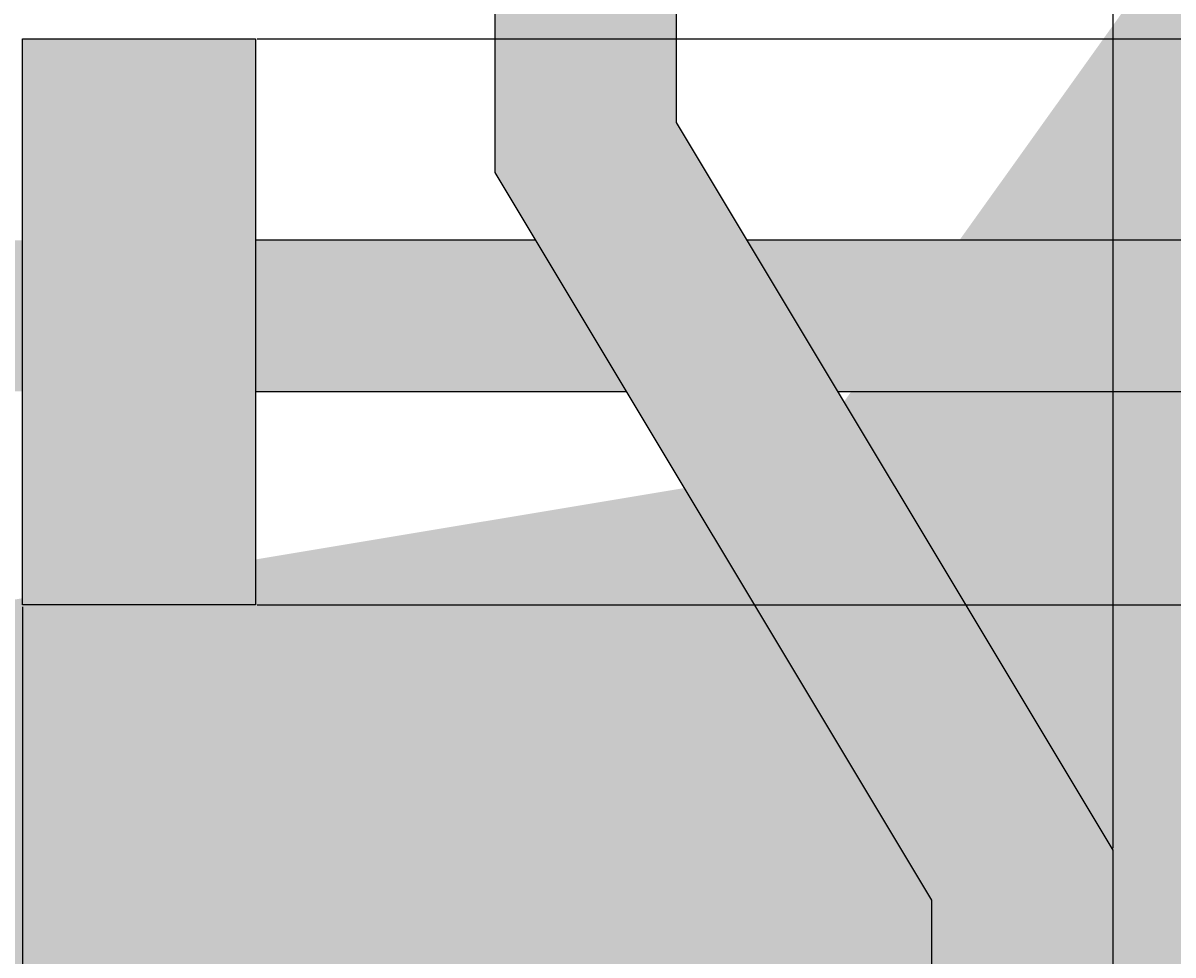
# Model space of a CAD drawing. Units: millimetres. Extents: x -22994 to 29398, y -19990 to 20176.
# Tile 111 of 135: x 166 to 204, y 124 to 155. Entities that reach past the tile are written whole.
import ezdxf

# ---------------------------------------------------------------- set-up
doc = ezdxf.new("R2010")
doc.units = ezdxf.units.MM
doc.header["$MEASUREMENT"] = 0
for name, color, linetype, lineweight in [('M-DIMS', 2, 'Continuous', 18), ('M-EQPM', 7, 'Continuous', 25), ('M-EQPM-PATT', 7, 'Continuous', 18)]:
    doc.layers.add(name, color=color, linetype=linetype, lineweight=lineweight)
doc.styles.get("Standard").update_dxf_attribs({"font": 'arial.ttf'})
doc.dimstyles.get("Standard").update_dxf_attribs({"dimtxt": 0.18, "dimasz": 10000, "dimexe": 0.18, "dimexo": 0.0625, "dimgap": 0.09, "dimtad": 0, "dimtih": 1, "dimtoh": 1, "dimdec": 0, "dimzin": 0, "dimdsep": 46, "dimtxsty": 'Standard', "dimcen": 0.09, "dimadec": 0, "dimazin": 0, "dimtfac": 1, "dimtdec": 0, "dimtofl": 0, "dimtmove": 0, "dimatfit": 3, "dimfxl": 1, "dimtolj": 1, "dimtzin": 0, "dimlwd": 30, "dimarcsym": 0})

# ---------------------------------------------------------------- blocks, each defined once
blk = doc.blocks.new('*D2')
at = {"layer": 'Defpoints', "color": 0, "transparency": 16777216}
for p in [(6.677, 10.271), (290.852, 10.271), (290.852, -5.079)]:
    blk.add_point(p, dxfattribs=at)
at = {"layer": 'M-DIMS', "color": 0, "lineweight": -2, "transparency": 16777216}
for p, q in [((6.677, 10.209), (6.677, -5.259)), ((290.852, 10.209), (290.852, -5.259))]:
    blk.add_line(p, q, dxfattribs=at)
at = {"layer": 'M-DIMS', "color": 0, "lineweight": 30, "transparency": 16777216}
for p, q in [((-9993.323, -5.079), (-19993.323, -5.079)), ((10290.852, -5.079), (20290.852, -5.079))]:
    blk.add_line(p, q, dxfattribs=at)
at = {"layer": 'M-DIMS', "color": 0, "transparency": 16777216}
for points in [[(-9993.323, 1661.588), (-9993.323, -1671.745), (6.677, -5.079)], [(10290.852, 1661.588), (10290.852, -1671.745), (290.852, -5.079)]]:
    blk.add_solid(points, dxfattribs=at)
at = {"layer": 'M-DIMS', "color": 0, "transparency": 16777216, "insert": (148.765, -5.079), "char_height": 0.18, "attachment_point": 5}
blk.add_mtext('\\A1;284.2', dxfattribs=at)
blk = doc.blocks.new('*D3')
at = {"layer": 'Defpoints', "color": 0, "transparency": 16777216}
for p in [(110.265, 204.165), (110.265, 176.366), (95.833, 127.967)]:
    blk.add_point(p, dxfattribs=at)
at = {"layer": 'M-DIMS', "color": 0, "lineweight": 30, "transparency": 16777216}
for p, q in [((-9904.167, 204.165), (-19904.167, 204.165)), ((10110.265, 204.165), (20110.265, 204.165))]:
    blk.add_line(p, q, dxfattribs=at)
at = {"layer": 'M-DIMS', "color": 0, "lineweight": -2, "transparency": 16777216}
for p, q in [((95.833, 128.03), (95.833, 204.345)), ((110.265, 176.429), (110.265, 204.345))]:
    blk.add_line(p, q, dxfattribs=at)
at = {"layer": 'M-DIMS', "color": 0, "transparency": 16777216}
for points in [[(-9904.167, 1870.832), (-9904.167, -1462.501), (95.833, 204.165)], [(10110.265, 1870.832), (10110.265, -1462.501), (110.265, 204.165)]]:
    blk.add_solid(points, dxfattribs=at)
at = {"layer": 'M-DIMS', "color": 0, "transparency": 16777216, "insert": (103.049, 204.165), "char_height": 0.18, "attachment_point": 5}
blk.add_mtext('\\A1;14.432', dxfattribs=at)
blk = doc.blocks.new('*D4')
at = {"layer": 'Defpoints', "color": 0, "transparency": 16777216}
for p in [(116.265, 204.165), (110.265, 176.366), (116.265, 176.366)]:
    blk.add_point(p, dxfattribs=at)
at = {"layer": 'M-DIMS', "color": 0, "lineweight": 30, "transparency": 16777216}
for p, q in [((-9889.735, 204.165), (-19889.735, 204.165)), ((10116.265, 204.165), (20116.265, 204.165))]:
    blk.add_line(p, q, dxfattribs=at)
at = {"layer": 'M-DIMS', "color": 0, "lineweight": -2, "transparency": 16777216}
for p, q in [((110.265, 176.429), (110.265, 204.345)), ((116.265, 176.429), (116.265, 204.345))]:
    blk.add_line(p, q, dxfattribs=at)
at = {"layer": 'M-DIMS', "color": 0, "transparency": 16777216}
for points in [[(-9889.735, 1870.832), (-9889.735, -1462.501), (110.265, 204.165)], [(10116.265, 1870.832), (10116.265, -1462.501), (116.265, 204.165)]]:
    blk.add_solid(points, dxfattribs=at)
at = {"layer": 'M-DIMS', "color": 0, "transparency": 16777216, "insert": (113.265, 204.165), "char_height": 0.18, "attachment_point": 5}
blk.add_mtext('\\A1;6', dxfattribs=at)
blk = doc.blocks.new('*D5')
at = {"layer": 'Defpoints', "color": 0, "transparency": 16777216}
for p in [(181.265, 204.165), (116.265, 176.366), (181.265, 176.366)]:
    blk.add_point(p, dxfattribs=at)
at = {"layer": 'M-DIMS', "color": 0, "lineweight": 30, "transparency": 16777216}
for p, q in [((-9883.735, 204.165), (-19883.735, 204.165)), ((10181.265, 204.165), (20181.265, 204.165))]:
    blk.add_line(p, q, dxfattribs=at)
at = {"layer": 'M-DIMS', "color": 0, "lineweight": -2, "transparency": 16777216}
for p, q in [((116.265, 176.429), (116.265, 204.345)), ((181.265, 176.429), (181.265, 204.345))]:
    blk.add_line(p, q, dxfattribs=at)
at = {"layer": 'M-DIMS', "color": 0, "transparency": 16777216}
for points in [[(-9883.735, 1870.832), (-9883.735, -1462.501), (116.265, 204.165)], [(10181.265, 1870.832), (10181.265, -1462.501), (181.265, 204.165)]]:
    blk.add_solid(points, dxfattribs=at)
at = {"layer": 'M-DIMS', "color": 0, "transparency": 16777216, "insert": (148.765, 204.165), "char_height": 0.18, "attachment_point": 5}
blk.add_mtext('\\A1;65', dxfattribs=at)
blk = doc.blocks.new('*D6')
at = {"layer": 'Defpoints', "color": 0, "transparency": 16777216}
for p in [(187.265, 204.165), (181.265, 176.366), (187.265, 176.366)]:
    blk.add_point(p, dxfattribs=at)
at = {"layer": 'M-DIMS', "color": 0, "lineweight": 30, "transparency": 16777216}
for p, q in [((-9818.735, 204.165), (-19818.735, 204.165)), ((10187.265, 204.165), (20187.265, 204.165))]:
    blk.add_line(p, q, dxfattribs=at)
at = {"layer": 'M-DIMS', "color": 0, "lineweight": -2, "transparency": 16777216}
for p, q in [((181.265, 176.429), (181.265, 204.345)), ((187.265, 176.429), (187.265, 204.345))]:
    blk.add_line(p, q, dxfattribs=at)
at = {"layer": 'M-DIMS', "color": 0, "transparency": 16777216}
for points in [[(-9818.735, 1870.832), (-9818.735, -1462.501), (181.265, 204.165)], [(10187.265, 1870.832), (10187.265, -1462.501), (187.265, 204.165)]]:
    blk.add_solid(points, dxfattribs=at)
at = {"layer": 'M-DIMS', "color": 0, "transparency": 16777216, "insert": (184.265, 204.165), "char_height": 0.18, "attachment_point": 5}
blk.add_mtext('\\A1;6', dxfattribs=at)
blk = doc.blocks.new('*D7')
at = {"layer": 'Defpoints', "color": 0, "transparency": 16777216}
for p in [(201.697, 204.165), (187.265, 176.366), (201.697, 127.967)]:
    blk.add_point(p, dxfattribs=at)
at = {"layer": 'M-DIMS', "color": 0, "lineweight": 30, "transparency": 16777216}
for p, q in [((-9812.735, 204.165), (-19812.735, 204.165)), ((10201.697, 204.165), (20201.697, 204.165))]:
    blk.add_line(p, q, dxfattribs=at)
at = {"layer": 'M-DIMS', "color": 0, "lineweight": -2, "transparency": 16777216}
for p, q in [((187.265, 176.429), (187.265, 204.345)), ((201.697, 128.03), (201.697, 204.345))]:
    blk.add_line(p, q, dxfattribs=at)
at = {"layer": 'M-DIMS', "color": 0, "transparency": 16777216}
for points in [[(-9812.735, 1870.832), (-9812.735, -1462.501), (187.265, 204.165)], [(10201.697, 1870.832), (10201.697, -1462.501), (201.697, 204.165)]]:
    blk.add_solid(points, dxfattribs=at)
at = {"layer": 'M-DIMS', "color": 0, "transparency": 16777216, "insert": (194.481, 204.165), "char_height": 0.18, "attachment_point": 5}
blk.add_mtext('\\A1;14.432', dxfattribs=at)
blk = doc.blocks.new('*D8')
at = {"layer": 'Defpoints', "color": 0, "transparency": 16777216}
for p in [(227.648, 204.165), (227.648, 146.73), (201.697, 127.967)]:
    blk.add_point(p, dxfattribs=at)
at = {"layer": 'M-DIMS', "color": 0, "lineweight": 30, "transparency": 16777216}
for p, q in [((-9798.303, 204.165), (-19798.303, 204.165)), ((10227.648, 204.165), (20227.648, 204.165))]:
    blk.add_line(p, q, dxfattribs=at)
at = {"layer": 'M-DIMS', "color": 0, "lineweight": -2, "transparency": 16777216}
for p, q in [((201.697, 128.03), (201.697, 204.345)), ((227.648, 146.792), (227.648, 204.345))]:
    blk.add_line(p, q, dxfattribs=at)
at = {"layer": 'M-DIMS', "color": 0, "transparency": 16777216}
for points in [[(-9798.303, 1870.832), (-9798.303, -1462.501), (201.697, 204.165)], [(10227.648, 1870.832), (10227.648, -1462.501), (227.648, 204.165)]]:
    blk.add_solid(points, dxfattribs=at)
at = {"layer": 'M-DIMS', "color": 0, "transparency": 16777216, "insert": (214.673, 204.165), "char_height": 0.18, "attachment_point": 5}
blk.add_mtext('\\A1;25.95', dxfattribs=at)
blk = doc.blocks.new('*D9')
at = {"layer": 'Defpoints', "color": 0, "transparency": 16777216}
for p in [(187.265, 176.366), (306.202, 176.366), (290.852, 10.271)]:
    blk.add_point(p, dxfattribs=at)
at = {"layer": 'M-DIMS', "color": 0, "lineweight": 30, "transparency": 16777216}
for p, q in [((306.202, 10176.366), (306.202, 20176.366)), ((306.202, -9989.729), (306.202, -19989.729))]:
    blk.add_line(p, q, dxfattribs=at)
at = {"layer": 'M-DIMS', "color": 0, "lineweight": -2, "transparency": 16777216}
for p, q in [((187.327, 176.366), (306.382, 176.366)), ((290.915, 10.271), (306.382, 10.271))]:
    blk.add_line(p, q, dxfattribs=at)
at = {"layer": 'M-DIMS', "color": 0, "transparency": 16777216}
for points in [[(-1360.465, 10176.366), (1972.869, 10176.366), (306.202, 176.366)], [(-1360.465, -9989.729), (1972.869, -9989.729), (306.202, 10.271)]]:
    blk.add_solid(points, dxfattribs=at)
at = {"layer": 'M-DIMS', "color": 0, "transparency": 16777216, "insert": (306.202, 93.319), "char_height": 0.18, "attachment_point": 5}
blk.add_mtext('\\A1;166.1', dxfattribs=at)
blk = doc.blocks.new('*D10')
at = {"layer": 'Defpoints', "color": 0, "transparency": 16777216}
for p in [(125.65, 136.071), (133.346, 136.071), (133.346, -5.079)]:
    blk.add_point(p, dxfattribs=at)
at = {"layer": 'M-DIMS', "color": 0, "lineweight": -2, "transparency": 16777216}
for p, q in [((125.65, 136.009), (125.65, -5.259)), ((133.346, 136.009), (133.346, -5.259))]:
    blk.add_line(p, q, dxfattribs=at)
at = {"layer": 'M-DIMS', "color": 0, "lineweight": 30, "transparency": 16777216}
for p, q in [((-9874.35, -5.079), (-19874.35, -5.079)), ((10133.346, -5.079), (20133.346, -5.079))]:
    blk.add_line(p, q, dxfattribs=at)
at = {"layer": 'M-DIMS', "color": 0, "transparency": 16777216}
for points in [[(-9874.35, 1661.588), (-9874.35, -1671.745), (125.65, -5.079)], [(10133.346, 1661.588), (10133.346, -1671.745), (133.346, -5.079)]]:
    blk.add_solid(points, dxfattribs=at)
at = {"layer": 'M-DIMS', "color": 0, "transparency": 16777216, "insert": (129.498, -5.079), "char_height": 0.18, "attachment_point": 5}
blk.add_mtext('\\A1;7.696', dxfattribs=at)
blk = doc.blocks.new('*D11')
at = {"layer": 'Defpoints', "color": 0, "transparency": 16777216}
for p in [(133.346, 136.071), (135.65, 136.071), (135.65, -5.079)]:
    blk.add_point(p, dxfattribs=at)
at = {"layer": 'M-DIMS', "color": 0, "lineweight": -2, "transparency": 16777216}
for p, q in [((133.346, 136.009), (133.346, -5.259)), ((135.65, 136.009), (135.65, -5.259))]:
    blk.add_line(p, q, dxfattribs=at)
at = {"layer": 'M-DIMS', "color": 0, "lineweight": 30, "transparency": 16777216}
for p, q in [((-9866.654, -5.079), (-19866.654, -5.079)), ((10135.65, -5.079), (20135.65, -5.079))]:
    blk.add_line(p, q, dxfattribs=at)
at = {"layer": 'M-DIMS', "color": 0, "transparency": 16777216}
for points in [[(-9866.654, 1661.588), (-9866.654, -1671.745), (133.346, -5.079)], [(10135.65, 1661.588), (10135.65, -1671.745), (135.65, -5.079)]]:
    blk.add_solid(points, dxfattribs=at)
at = {"layer": 'M-DIMS', "color": 0, "transparency": 16777216, "insert": (134.498, -5.079), "char_height": 0.18, "attachment_point": 5}
blk.add_mtext('\\A1;2.304', dxfattribs=at)
blk = doc.blocks.new('*D12')
at = {"layer": 'Defpoints', "color": 0, "transparency": 16777216}
for p in [(135.65, 136.071), (145.65, 136.071), (145.65, -5.079)]:
    blk.add_point(p, dxfattribs=at)
at = {"layer": 'M-DIMS', "color": 0, "lineweight": -2, "transparency": 16777216}
for p, q in [((135.65, 136.009), (135.65, -5.259)), ((145.65, 136.009), (145.65, -5.259))]:
    blk.add_line(p, q, dxfattribs=at)
at = {"layer": 'M-DIMS', "color": 0, "lineweight": 30, "transparency": 16777216}
for p, q in [((-9864.35, -5.079), (-19864.35, -5.079)), ((10145.65, -5.079), (20145.65, -5.079))]:
    blk.add_line(p, q, dxfattribs=at)
at = {"layer": 'M-DIMS', "color": 0, "transparency": 16777216}
for points in [[(-9864.35, 1661.588), (-9864.35, -1671.745), (135.65, -5.079)], [(10145.65, 1661.588), (10145.65, -1671.745), (145.65, -5.079)]]:
    blk.add_solid(points, dxfattribs=at)
at = {"layer": 'M-DIMS', "color": 0, "transparency": 16777216, "insert": (140.65, -5.079), "char_height": 0.18, "attachment_point": 5}
blk.add_mtext('\\A1;10', dxfattribs=at)
blk = doc.blocks.new('*D13')
at = {"layer": 'Defpoints', "color": 0, "transparency": 16777216}
for p in [(145.65, 136.071), (155.65, 136.071), (155.65, -5.079)]:
    blk.add_point(p, dxfattribs=at)
at = {"layer": 'M-DIMS', "color": 0, "lineweight": -2, "transparency": 16777216}
for p, q in [((145.65, 136.009), (145.65, -5.259)), ((155.65, 136.009), (155.65, -5.259))]:
    blk.add_line(p, q, dxfattribs=at)
at = {"layer": 'M-DIMS', "color": 0, "lineweight": 30, "transparency": 16777216}
for p, q in [((-9854.35, -5.079), (-19854.35, -5.079)), ((10155.65, -5.079), (20155.65, -5.079))]:
    blk.add_line(p, q, dxfattribs=at)
at = {"layer": 'M-DIMS', "color": 0, "transparency": 16777216}
for points in [[(-9854.35, 1661.588), (-9854.35, -1671.745), (145.65, -5.079)], [(10155.65, 1661.588), (10155.65, -1671.745), (155.65, -5.079)]]:
    blk.add_solid(points, dxfattribs=at)
at = {"layer": 'M-DIMS', "color": 0, "transparency": 16777216, "insert": (150.65, -5.079), "char_height": 0.18, "attachment_point": 5}
blk.add_mtext('\\A1;10', dxfattribs=at)
blk = doc.blocks.new('*D14')
at = {"layer": 'Defpoints', "color": 0, "transparency": 16777216}
for p in [(155.65, 136.071), (165.65, 136.071), (165.65, -5.079)]:
    blk.add_point(p, dxfattribs=at)
at = {"layer": 'M-DIMS', "color": 0, "lineweight": -2, "transparency": 16777216}
for p, q in [((155.65, 136.009), (155.65, -5.259)), ((165.65, 136.009), (165.65, -5.259))]:
    blk.add_line(p, q, dxfattribs=at)
at = {"layer": 'M-DIMS', "color": 0, "lineweight": 30, "transparency": 16777216}
for p, q in [((-9844.35, -5.079), (-19844.35, -5.079)), ((10165.65, -5.079), (20165.65, -5.079))]:
    blk.add_line(p, q, dxfattribs=at)
at = {"layer": 'M-DIMS', "color": 0, "transparency": 16777216}
for points in [[(-9844.35, 1661.588), (-9844.35, -1671.745), (155.65, -5.079)], [(10165.65, 1661.588), (10165.65, -1671.745), (165.65, -5.079)]]:
    blk.add_solid(points, dxfattribs=at)
at = {"layer": 'M-DIMS', "color": 0, "transparency": 16777216, "insert": (160.65, -5.079), "char_height": 0.18, "attachment_point": 5}
blk.add_mtext('\\A1;10', dxfattribs=at)
blk = doc.blocks.new('*D15')
at = {"layer": 'Defpoints', "color": 0, "transparency": 16777216}
for p in [(173.346, 154.788), (173.346, 136.071), (306.202, 136.071)]:
    blk.add_point(p, dxfattribs=at)
at = {"layer": 'M-DIMS', "color": 0, "lineweight": 30, "transparency": 16777216}
for p, q in [((306.202, 10154.788), (306.202, 20154.788)), ((306.202, -9863.929), (306.202, -19863.929))]:
    blk.add_line(p, q, dxfattribs=at)
at = {"layer": 'M-DIMS', "color": 0, "lineweight": -2, "transparency": 16777216}
for p, q in [((173.408, 154.788), (306.382, 154.788)), ((173.408, 136.071), (306.382, 136.071))]:
    blk.add_line(p, q, dxfattribs=at)
at = {"layer": 'M-DIMS', "color": 0, "transparency": 16777216}
for points in [[(-1360.465, 10154.788), (1972.869, 10154.788), (306.202, 154.788)], [(-1360.465, -9863.929), (1972.869, -9863.929), (306.202, 136.071)]]:
    blk.add_solid(points, dxfattribs=at)
at = {"layer": 'M-DIMS', "color": 0, "transparency": 16777216, "insert": (306.202, 145.43), "char_height": 0.18, "attachment_point": 5}
blk.add_mtext('\\A1;18.717', dxfattribs=at)
blk = doc.blocks.new('*D16')
at = {"layer": 'Defpoints', "color": 0, "transparency": 16777216}
for p in [(120.17, 204.165), (110.466, 48.035), (120.17, 48.035)]:
    blk.add_point(p, dxfattribs=at)
at = {"layer": 'M-DIMS', "color": 0, "lineweight": 30, "transparency": 16777216}
for p, q in [((-9889.534, 204.165), (-19889.534, 204.165)), ((10120.17, 204.165), (20120.17, 204.165))]:
    blk.add_line(p, q, dxfattribs=at)
at = {"layer": 'M-DIMS', "color": 0, "lineweight": -2, "transparency": 16777216}
for p, q in [((110.466, 48.097), (110.466, 204.345)), ((120.17, 48.097), (120.17, 204.345))]:
    blk.add_line(p, q, dxfattribs=at)
at = {"layer": 'M-DIMS', "color": 0, "transparency": 16777216}
for points in [[(-9889.534, 1870.832), (-9889.534, -1462.501), (110.466, 204.165)], [(10120.17, 1870.832), (10120.17, -1462.501), (120.17, 204.165)]]:
    blk.add_solid(points, dxfattribs=at)
at = {"layer": 'M-DIMS', "color": 0, "transparency": 16777216, "insert": (115.318, 204.165), "char_height": 0.18, "attachment_point": 5}
blk.add_mtext('\\A1;9.704', dxfattribs=at)
blk = doc.blocks.new('*D17')
at = {"layer": 'Defpoints', "color": 0, "transparency": 16777216}
for p in [(126.17, 204.165), (120.17, 48.035), (126.17, 48.035)]:
    blk.add_point(p, dxfattribs=at)
at = {"layer": 'M-DIMS', "color": 0, "lineweight": 30, "transparency": 16777216}
for p, q in [((-9879.83, 204.165), (-19879.83, 204.165)), ((10126.17, 204.165), (20126.17, 204.165))]:
    blk.add_line(p, q, dxfattribs=at)
at = {"layer": 'M-DIMS', "color": 0, "lineweight": -2, "transparency": 16777216}
for p, q in [((120.17, 48.097), (120.17, 204.345)), ((126.17, 48.097), (126.17, 204.345))]:
    blk.add_line(p, q, dxfattribs=at)
at = {"layer": 'M-DIMS', "color": 0, "transparency": 16777216}
for points in [[(-9879.83, 1870.832), (-9879.83, -1462.501), (120.17, 204.165)], [(10126.17, 1870.832), (10126.17, -1462.501), (126.17, 204.165)]]:
    blk.add_solid(points, dxfattribs=at)
at = {"layer": 'M-DIMS', "color": 0, "transparency": 16777216, "insert": (123.17, 204.165), "char_height": 0.18, "attachment_point": 5}
blk.add_mtext('\\A1;6', dxfattribs=at)
blk = doc.blocks.new('*D18')
at = {"layer": 'Defpoints', "color": 0, "transparency": 16777216}
for p in [(132.17, 204.165), (126.17, 48.035), (132.17, 48.035)]:
    blk.add_point(p, dxfattribs=at)
at = {"layer": 'M-DIMS', "color": 0, "lineweight": 30, "transparency": 16777216}
for p, q in [((-9873.83, 204.165), (-19873.83, 204.165)), ((10132.17, 204.165), (20132.17, 204.165))]:
    blk.add_line(p, q, dxfattribs=at)
at = {"layer": 'M-DIMS', "color": 0, "lineweight": -2, "transparency": 16777216}
for p, q in [((126.17, 48.097), (126.17, 204.345)), ((132.17, 48.097), (132.17, 204.345))]:
    blk.add_line(p, q, dxfattribs=at)
at = {"layer": 'M-DIMS', "color": 0, "transparency": 16777216}
for points in [[(-9873.83, 1870.832), (-9873.83, -1462.501), (126.17, 204.165)], [(10132.17, 1870.832), (10132.17, -1462.501), (132.17, 204.165)]]:
    blk.add_solid(points, dxfattribs=at)
at = {"layer": 'M-DIMS', "color": 0, "transparency": 16777216, "insert": (129.17, 204.165), "char_height": 0.18, "attachment_point": 5}
blk.add_mtext('\\A1;6', dxfattribs=at)
blk = doc.blocks.new('*D19')
at = {"layer": 'Defpoints', "color": 0, "transparency": 16777216}
for p in [(138.17, 204.165), (132.17, 48.035), (138.17, 48.035)]:
    blk.add_point(p, dxfattribs=at)
at = {"layer": 'M-DIMS', "color": 0, "lineweight": 30, "transparency": 16777216}
for p, q in [((-9867.83, 204.165), (-19867.83, 204.165)), ((10138.17, 204.165), (20138.17, 204.165))]:
    blk.add_line(p, q, dxfattribs=at)
at = {"layer": 'M-DIMS', "color": 0, "lineweight": -2, "transparency": 16777216}
for p, q in [((132.17, 48.097), (132.17, 204.345)), ((138.17, 48.097), (138.17, 204.345))]:
    blk.add_line(p, q, dxfattribs=at)
at = {"layer": 'M-DIMS', "color": 0, "transparency": 16777216}
for points in [[(-9867.83, 1870.832), (-9867.83, -1462.501), (132.17, 204.165)], [(10138.17, 1870.832), (10138.17, -1462.501), (138.17, 204.165)]]:
    blk.add_solid(points, dxfattribs=at)
at = {"layer": 'M-DIMS', "color": 0, "transparency": 16777216, "insert": (135.17, 204.165), "char_height": 0.18, "attachment_point": 5}
blk.add_mtext('\\A1;6', dxfattribs=at)
blk = doc.blocks.new('*D20')
at = {"layer": 'Defpoints', "color": 0, "transparency": 16777216}
for p in [(144.17, 204.165), (138.17, 48.035), (144.17, 48.035)]:
    blk.add_point(p, dxfattribs=at)
at = {"layer": 'M-DIMS', "color": 0, "lineweight": 30, "transparency": 16777216}
for p, q in [((-9861.83, 204.165), (-19861.83, 204.165)), ((10144.17, 204.165), (20144.17, 204.165))]:
    blk.add_line(p, q, dxfattribs=at)
at = {"layer": 'M-DIMS', "color": 0, "lineweight": -2, "transparency": 16777216}
for p, q in [((138.17, 48.097), (138.17, 204.345)), ((144.17, 48.097), (144.17, 204.345))]:
    blk.add_line(p, q, dxfattribs=at)
at = {"layer": 'M-DIMS', "color": 0, "transparency": 16777216}
for points in [[(-9861.83, 1870.832), (-9861.83, -1462.501), (138.17, 204.165)], [(10144.17, 1870.832), (10144.17, -1462.501), (144.17, 204.165)]]:
    blk.add_solid(points, dxfattribs=at)
at = {"layer": 'M-DIMS', "color": 0, "transparency": 16777216, "insert": (141.17, 204.165), "char_height": 0.18, "attachment_point": 5}
blk.add_mtext('\\A1;6', dxfattribs=at)
blk = doc.blocks.new('*D21')
at = {"layer": 'Defpoints', "color": 0, "transparency": 16777216}
for p in [(149.116, 204.165), (144.17, 48.035), (149.116, 48.035)]:
    blk.add_point(p, dxfattribs=at)
at = {"layer": 'M-DIMS', "color": 0, "lineweight": 30, "transparency": 16777216}
for p, q in [((-9855.83, 204.165), (-19855.83, 204.165)), ((10149.116, 204.165), (20149.116, 204.165))]:
    blk.add_line(p, q, dxfattribs=at)
at = {"layer": 'M-DIMS', "color": 0, "lineweight": -2, "transparency": 16777216}
for p, q in [((144.17, 48.097), (144.17, 204.345)), ((149.116, 48.097), (149.116, 204.345))]:
    blk.add_line(p, q, dxfattribs=at)
at = {"layer": 'M-DIMS', "color": 0, "transparency": 16777216}
for points in [[(-9855.83, 1870.832), (-9855.83, -1462.501), (144.17, 204.165)], [(10149.116, 1870.832), (10149.116, -1462.501), (149.116, 204.165)]]:
    blk.add_solid(points, dxfattribs=at)
at = {"layer": 'M-DIMS', "color": 0, "transparency": 16777216, "insert": (146.643, 204.165), "char_height": 0.18, "attachment_point": 5}
blk.add_mtext('\\A1;4.945', dxfattribs=at)
blk = doc.blocks.new('*D22')
at = {"layer": 'Defpoints', "color": 0, "transparency": 16777216}
for p in [(149.116, 30.99), (155.116, 30.99), (155.116, -5.079)]:
    blk.add_point(p, dxfattribs=at)
at = {"layer": 'M-DIMS', "color": 0, "lineweight": -2, "transparency": 16777216}
for p, q in [((149.116, 30.927), (149.116, -5.259)), ((155.116, 30.927), (155.116, -5.259))]:
    blk.add_line(p, q, dxfattribs=at)
at = {"layer": 'M-DIMS', "color": 0, "lineweight": 30, "transparency": 16777216}
for p, q in [((-9850.884, -5.079), (-19850.884, -5.079)), ((10155.116, -5.079), (20155.116, -5.079))]:
    blk.add_line(p, q, dxfattribs=at)
at = {"layer": 'M-DIMS', "color": 0, "transparency": 16777216}
for points in [[(-9850.884, 1661.588), (-9850.884, -1671.745), (149.116, -5.079)], [(10155.116, 1661.588), (10155.116, -1671.745), (155.116, -5.079)]]:
    blk.add_solid(points, dxfattribs=at)
at = {"layer": 'M-DIMS', "color": 0, "transparency": 16777216, "insert": (152.116, -5.079), "char_height": 0.18, "attachment_point": 5}
blk.add_mtext('\\A1;6', dxfattribs=at)
blk = doc.blocks.new('*D23')
at = {"layer": 'Defpoints', "color": 0, "transparency": 16777216}
for p in [(155.116, 30.99), (161.116, 30.99), (161.116, -5.079)]:
    blk.add_point(p, dxfattribs=at)
at = {"layer": 'M-DIMS', "color": 0, "lineweight": -2, "transparency": 16777216}
for p, q in [((155.116, 30.927), (155.116, -5.259)), ((161.116, 30.927), (161.116, -5.259))]:
    blk.add_line(p, q, dxfattribs=at)
at = {"layer": 'M-DIMS', "color": 0, "lineweight": 30, "transparency": 16777216}
for p, q in [((-9844.884, -5.079), (-19844.884, -5.079)), ((10161.116, -5.079), (20161.116, -5.079))]:
    blk.add_line(p, q, dxfattribs=at)
at = {"layer": 'M-DIMS', "color": 0, "transparency": 16777216}
for points in [[(-9844.884, 1661.588), (-9844.884, -1671.745), (155.116, -5.079)], [(10161.116, 1661.588), (10161.116, -1671.745), (161.116, -5.079)]]:
    blk.add_solid(points, dxfattribs=at)
at = {"layer": 'M-DIMS', "color": 0, "transparency": 16777216, "insert": (158.116, -5.079), "char_height": 0.18, "attachment_point": 5}
blk.add_mtext('\\A1;6', dxfattribs=at)
blk = doc.blocks.new('*D24')
at = {"layer": 'Defpoints', "color": 0, "transparency": 16777216}
for p in [(161.116, 30.99), (166.439, 30.99), (166.439, -5.079)]:
    blk.add_point(p, dxfattribs=at)
at = {"layer": 'M-DIMS', "color": 0, "lineweight": -2, "transparency": 16777216}
for p, q in [((161.116, 30.927), (161.116, -5.259)), ((166.439, 30.927), (166.439, -5.259))]:
    blk.add_line(p, q, dxfattribs=at)
at = {"layer": 'M-DIMS', "color": 0, "lineweight": 30, "transparency": 16777216}
for p, q in [((-9838.884, -5.079), (-19838.884, -5.079)), ((10166.439, -5.079), (20166.439, -5.079))]:
    blk.add_line(p, q, dxfattribs=at)
at = {"layer": 'M-DIMS', "color": 0, "transparency": 16777216}
for points in [[(-9838.884, 1661.588), (-9838.884, -1671.745), (161.116, -5.079)], [(10166.439, 1661.588), (10166.439, -1671.745), (166.439, -5.079)]]:
    blk.add_solid(points, dxfattribs=at)
at = {"layer": 'M-DIMS', "color": 0, "transparency": 16777216, "insert": (163.777, -5.079), "char_height": 0.18, "attachment_point": 5}
blk.add_mtext('\\A1;5.323', dxfattribs=at)
blk = doc.blocks.new('*D25')
at = {"layer": 'Defpoints', "color": 0, "transparency": 16777216}
for p in [(166.439, 30.99), (172.439, 30.99), (172.439, -5.079)]:
    blk.add_point(p, dxfattribs=at)
at = {"layer": 'M-DIMS', "color": 0, "lineweight": -2, "transparency": 16777216}
for p, q in [((166.439, 30.927), (166.439, -5.259)), ((172.439, 30.927), (172.439, -5.259))]:
    blk.add_line(p, q, dxfattribs=at)
at = {"layer": 'M-DIMS', "color": 0, "lineweight": 30, "transparency": 16777216}
for p, q in [((-9833.561, -5.079), (-19833.561, -5.079)), ((10172.439, -5.079), (20172.439, -5.079))]:
    blk.add_line(p, q, dxfattribs=at)
at = {"layer": 'M-DIMS', "color": 0, "transparency": 16777216}
for points in [[(-9833.561, 1661.588), (-9833.561, -1671.745), (166.439, -5.079)], [(10172.439, 1661.588), (10172.439, -1671.745), (172.439, -5.079)]]:
    blk.add_solid(points, dxfattribs=at)
at = {"layer": 'M-DIMS', "color": 0, "transparency": 16777216, "insert": (169.439, -5.079), "char_height": 0.18, "attachment_point": 5}
blk.add_mtext('\\A1;6', dxfattribs=at)
blk = doc.blocks.new('*D26')
at = {"layer": 'Defpoints', "color": 0, "transparency": 16777216}
for p in [(172.439, 30.99), (178.439, 30.99), (178.439, -5.079)]:
    blk.add_point(p, dxfattribs=at)
at = {"layer": 'M-DIMS', "color": 0, "lineweight": -2, "transparency": 16777216}
for p, q in [((172.439, 30.927), (172.439, -5.259)), ((178.439, 30.927), (178.439, -5.259))]:
    blk.add_line(p, q, dxfattribs=at)
at = {"layer": 'M-DIMS', "color": 0, "lineweight": 30, "transparency": 16777216}
for p, q in [((-9827.561, -5.079), (-19827.561, -5.079)), ((10178.439, -5.079), (20178.439, -5.079))]:
    blk.add_line(p, q, dxfattribs=at)
at = {"layer": 'M-DIMS', "color": 0, "transparency": 16777216}
for points in [[(-9827.561, 1661.588), (-9827.561, -1671.745), (172.439, -5.079)], [(10178.439, 1661.588), (10178.439, -1671.745), (178.439, -5.079)]]:
    blk.add_solid(points, dxfattribs=at)
at = {"layer": 'M-DIMS', "color": 0, "transparency": 16777216, "insert": (175.439, -5.079), "char_height": 0.18, "attachment_point": 5}
blk.add_mtext('\\A1;6', dxfattribs=at)
blk = doc.blocks.new('*D27')
at = {"layer": 'Defpoints', "color": 0, "transparency": 16777216}
for p in [(178.439, 30.99), (188.117, 30.99), (188.117, -5.079)]:
    blk.add_point(p, dxfattribs=at)
at = {"layer": 'M-DIMS', "color": 0, "lineweight": -2, "transparency": 16777216}
for p, q in [((178.439, 30.927), (178.439, -5.259)), ((188.117, 30.927), (188.117, -5.259))]:
    blk.add_line(p, q, dxfattribs=at)
at = {"layer": 'M-DIMS', "color": 0, "lineweight": 30, "transparency": 16777216}
for p, q in [((-9821.561, -5.079), (-19821.561, -5.079)), ((10188.117, -5.079), (20188.117, -5.079))]:
    blk.add_line(p, q, dxfattribs=at)
at = {"layer": 'M-DIMS', "color": 0, "transparency": 16777216}
for points in [[(-9821.561, 1661.588), (-9821.561, -1671.745), (178.439, -5.079)], [(10188.117, 1661.588), (10188.117, -1671.745), (188.117, -5.079)]]:
    blk.add_solid(points, dxfattribs=at)
at = {"layer": 'M-DIMS', "color": 0, "transparency": 16777216, "insert": (183.278, -5.079), "char_height": 0.18, "attachment_point": 5}
blk.add_mtext('\\A1;9.679', dxfattribs=at)
blk = doc.blocks.new('*D28')
at = {"layer": 'Defpoints', "color": 0, "transparency": 16777216}
for p in [(188.117, 48.035), (306.202, 48.035), (188.117, 30.99)]:
    blk.add_point(p, dxfattribs=at)
at = {"layer": 'M-DIMS', "color": 0, "lineweight": 30, "transparency": 16777216}
for p, q in [((306.202, 10048.035), (306.202, 20048.035)), ((306.202, -9969.01), (306.202, -19969.01))]:
    blk.add_line(p, q, dxfattribs=at)
at = {"layer": 'M-DIMS', "color": 0, "lineweight": -2, "transparency": 16777216}
for p, q in [((188.18, 48.035), (306.382, 48.035)), ((188.18, 30.99), (306.382, 30.99))]:
    blk.add_line(p, q, dxfattribs=at)
at = {"layer": 'M-DIMS', "color": 0, "transparency": 16777216}
for points in [[(-1360.465, 10048.035), (1972.869, 10048.035), (306.202, 48.035)], [(-1360.465, -9969.01), (1972.869, -9969.01), (306.202, 30.99)]]:
    blk.add_solid(points, dxfattribs=at)
at = {"layer": 'M-DIMS', "color": 0, "transparency": 16777216, "insert": (306.202, 39.512), "char_height": 0.18, "attachment_point": 5}
blk.add_mtext('\\A1;17.045', dxfattribs=at)
blk = doc.blocks.new('*D29')
at = {"layer": 'Defpoints', "color": 0, "transparency": 16777216}
for p in [(36.801, 80.045), (64.03, 80.045)]:
    blk.add_point(p, dxfattribs=at)
at = {"layer": 'M-DIMS', "color": 0, "lineweight": -2, "transparency": 16777216}
for p, q in [((50.325, 80.045), (50.505, 80.045)), ((50.415, 79.955), (50.415, 80.135))]:
    blk.add_line(p, q, dxfattribs=at)
at = {"layer": 'M-DIMS', "color": 0, "lineweight": 30, "transparency": 16777216}
blk.add_line((20064.03, 80.03), (10064.03, 80.038), dxfattribs=at)
at = {"layer": 'M-DIMS', "color": 0, "transparency": 16777216}
blk.add_solid([(10064.031, 1746.704), (10064.028, -1586.629), (64.03, 80.045)], dxfattribs=at)
at = {"layer": 'M-DIMS', "color": 0, "transparency": 16777216, "insert": (20064.521, 80.03), "char_height": 0.18, "attachment_point": 5}
blk.add_mtext('\\A1;∅27.23', dxfattribs=at)
blk = doc.blocks.new('*D34')
at = {"layer": 'Defpoints', "color": 0, "transparency": 16777216}
for p in [(178.58, 122.895), (176.812, 121.128)]:
    blk.add_point(p, dxfattribs=at)
at = {"layer": 'M-DIMS', "color": 0, "lineweight": 30, "transparency": 16777216}
for p, q in [((14322.436, 14263.311), (7250.508, 7193.103)), ((24322.436, 14263.311), (14322.436, 14263.311))]:
    blk.add_line(p, q, dxfattribs=at)
at = {"layer": 'M-DIMS', "color": 0, "lineweight": -2, "transparency": 16777216}
for p, q in [((176.722, 121.128), (176.902, 121.128)), ((176.812, 121.038), (176.812, 121.218))]:
    blk.add_line(p, q, dxfattribs=at)
at = {"layer": 'M-DIMS', "color": 0, "transparency": 16777216}
blk.add_solid([(6072.14, 8371.758), (8428.876, 6014.448), (178.58, 122.895)], dxfattribs=at)
at = {"layer": 'M-DIMS', "color": 0, "transparency": 16777216, "insert": (24322.97, 14263.311), "char_height": 0.18, "attachment_point": 5}
blk.add_mtext('\\A1;6X R2.5', dxfattribs=at)
blk = doc.blocks.new('*D36')
at = {"layer": 'Defpoints', "color": 0, "transparency": 16777216}
for p in [(46.39, 31.303), (46.387, 26.593)]:
    blk.add_point(p, dxfattribs=at)
at = {"layer": 'M-DIMS', "color": 0, "lineweight": 30, "transparency": 16777216}
for p, q in [((57.15, 20031.301), (51.77, 10031.302)), ((10057.15, 20031.301), (57.15, 20031.301))]:
    blk.add_line(p, q, dxfattribs=at)
at = {"layer": 'M-DIMS', "color": 0, "lineweight": -2, "transparency": 16777216}
for p, q in [((46.299, 28.948), (46.479, 28.948)), ((46.389, 28.858), (46.389, 29.038))]:
    blk.add_line(p, q, dxfattribs=at)
at = {"layer": 'M-DIMS', "color": 0, "transparency": 16777216}
blk.add_solid([(-1614.896, 10032.199), (1718.436, 10030.405), (46.39, 31.303)], dxfattribs=at)
at = {"layer": 'M-DIMS', "color": 0, "transparency": 16777216, "insert": (10057.554, 20031.301), "char_height": 0.18, "attachment_point": 5}
blk.add_mtext('\\A1;∅4.71', dxfattribs=at)
blk = doc.blocks.new('*D37')
at = {"layer": 'Defpoints', "color": 0, "transparency": 16777216}
for p in [(54.834, 118.615), (59.494, 118.614)]:
    blk.add_point(p, dxfattribs=at)
at = {"layer": 'M-DIMS', "color": 0, "lineweight": -2, "transparency": 16777216}
for p, q in [((57.074, 118.614), (57.254, 118.614)), ((57.164, 118.524), (57.164, 118.704))]:
    blk.add_line(p, q, dxfattribs=at)
at = {"layer": 'M-DIMS', "color": 0, "lineweight": 30, "transparency": 16777216}
blk.add_line((20059.493, 116.253), (10059.494, 117.434), dxfattribs=at)
at = {"layer": 'M-DIMS', "color": 0, "transparency": 16777216}
blk.add_solid([(10059.69, 1784.1), (10059.297, -1549.233), (59.494, 118.614)], dxfattribs=at)
at = {"layer": 'M-DIMS', "color": 0, "transparency": 16777216, "insert": (20059.985, 116.253), "char_height": 0.18, "attachment_point": 5}
blk.add_mtext('\\A1;∅4.659', dxfattribs=at)

msp = doc.modelspace()

# ---------------------------------------------------------------- hatches: boundary and pattern name
at = {"layer": 'M-EQPM-PATT'}
h = msp.add_hatch(color=256, dxfattribs=at)
h.set_gradient(color1=(205, 32, 39), color2=(205, 32, 39), tint=1)
h.paths.add_polyline_path([(116.2647, 150.3662), (116.2647, 170.3662), (116.2647, 176.3662), (110.2647, 176.3662), (110.2647, 152.0276), (95.8327, 127.967), (95.8327, 16.6063), (201.6967, 16.6063), (201.6967, 127.967), (187.2647, 152.0276), (187.2647, 176.3662), (181.2647, 176.3662), (181.2647, 170.3662), (181.2647, 150.3662), (195.6967, 126.3055), (195.6967, 22.6063), (101.8327, 22.6063), (101.8327, 126.3055)])
h.paths.add_polyline_path([(185.2208, 88.6347), (101.8327, 88.6347), (101.8327, 87.6347), (182.8066, 87.6347), (178.7313, 83.5594), (195.6967, 83.5594), (195.6967, 84.5594), (181.1455, 84.5594)], flags=17)
h.paths.add_polyline_path([(95.8327, 88.6347), (60.9779, 88.6347, -0.0228552), (61.7178, 87.6347), (95.8327, 87.6347)])
h.paths.add_polyline_path([(215.6212, 86.5189), (215.6212, 80.5999), (220.5095, 83.5594)])
h.paths.add_polyline_path([(215.6212, 84.5594), (201.6967, 84.5594), (201.6967, 83.5594), (215.6212, 83.5594)])
h.paths.add_polyline_path([(225.3978, 86.5189), (220.5095, 83.5594), (225.3978, 80.5999)])
h.paths.add_polyline_path([(231.6256, 84.5594), (225.3978, 84.5594), (225.3978, 83.5594), (231.6256, 83.5594)])
h = msp.add_hatch(color=256, dxfattribs=at)
h.set_gradient(color1=(128, 128, 128), color2=(128, 128, 128), tint=1)
h.paths.add_polyline_path([(88.0003, 148.1301), (88.0003, 143.1301), (104.9278, 143.1301), (107.9269, 148.1301)])
h.paths.add_polyline_path([(189.6025, 148.1301), (192.6016, 143.1301), (216.9016, 143.1301, -0.0809736), (216.3148, 146.7296, -0.0309822), (216.4017, 148.1301)])
h.paths.add_polyline_path([(229.9653, 167.6546), (245.0476, 167.6546), (245.0476, 172.6546), (224.9653, 172.6546), (224.9653, 157.741, -0.1116822), (229.9653, 157.8239)])
h.paths.add_polyline_path([(36.3887, 21.6644), (36.3887, 16.6063), (56.3887, 16.6063), (56.3887, 21.6644)])
h = msp.add_hatch(color=256, dxfattribs=at)
h.set_gradient(color1=(147, 39, 143), color2=(147, 39, 143), tint=1)
h.paths.add_polyline_path([(125.6498, 136.0713), (133.3459, 136.0713), (133.3459, 154.788), (125.6498, 154.788)])
h.paths.add_polyline_path([(135.6498, 136.0713), (143.3459, 136.0713), (143.3459, 154.788), (135.6498, 154.788)])
h.paths.add_polyline_path([(145.6498, 136.0713), (153.3459, 136.0713), (153.3459, 154.788), (145.6498, 154.788)])
h.paths.add_polyline_path([(155.6498, 136.0713), (163.3459, 136.0713), (163.3459, 154.788), (155.6498, 154.788)])
h.paths.add_polyline_path([(165.6498, 136.0713), (173.3459, 136.0713), (173.3459, 154.788), (165.6498, 154.788)])
h = msp.add_hatch(color=256, dxfattribs=at)
h.set_gradient(color1=(19, 155, 72), color2=(19, 155, 72), tint=1)
h.paths.add_polyline_path([(114.9234, 148.1301), (111.9243, 143.1301), (125.6498, 143.1301), (125.6498, 148.1301)])
h.paths.add_polyline_path([(173.3459, 148.1301), (173.3459, 143.1301), (185.605, 143.1301), (182.6059, 148.1301)])
h.paths.add_polyline_path([(135.6498, 148.1301), (133.3459, 148.1301), (133.3459, 143.1301), (135.6498, 143.1301)])
h.paths.add_polyline_path([(143.3459, 143.1301), (145.6498, 143.1301), (145.6498, 148.1301), (143.3459, 148.1301)])
h.paths.add_polyline_path([(153.3459, 143.1301), (155.6498, 143.1301), (155.6498, 148.1301), (153.3459, 148.1301)])
h.paths.add_polyline_path([(165.6498, 148.1301), (163.3459, 148.1301), (163.3459, 143.1301), (165.6498, 143.1301)])

# ---------------------------------------------------------------- linework, layer by layer
at = {"layer": 'M-EQPM'}
for p, q in [((182.6059, 148.1301), (173.3459, 148.1301)), ((216.4017, 148.1301), (189.6025, 148.1301)), ((173.3459, 143.1301), (185.605, 143.1301)), ((192.6016, 143.1301), (216.9016, 143.1301))]:
    msp.add_line(p, q, dxfattribs=at)
for points in [[(110.2647, 176.3662), (110.2647, 152.0276), (95.8327, 127.967), (95.8327, 16.6063), (201.6967, 16.6063), (201.6967, 127.967), (187.2647, 152.0276), (187.2647, 176.3662)], [(165.6498, 154.788), (173.3459, 154.788), (173.3459, 136.0713), (165.6498, 136.0713)]]:
    msp.add_lwpolyline(points, close=True, dxfattribs=at)
msp.add_lwpolyline([(116.2647, 170.3662), (116.2647, 150.3662), (101.8327, 126.3055), (101.8327, 22.6063), (195.6967, 22.6063), (195.6967, 126.3055), (181.2647, 150.3662), (181.2647, 170.3662)], dxfattribs=at)

# ---------------------------------------------------------------- dimensions: what is measured, and where the dimension line sits
at = {"layer": 'M-DIMS'}
for base, p1, p2, override, picture, middle in [((306.202, 176.3662), (290.852, 10.2713), (187.2647, 176.3662), {"dimdec": 1, "dimlfac": 1, "dimrnd": 0, "dimzin": 0, "dimdsep": 46, "dimlunit": 2}, '*D9', (306.202, 93.3187)), ((306.202, 136.0713), (173.3459, 154.788), (173.3459, 136.0713), {"dimdec": 3, "dimlfac": 1, "dimrnd": 0, "dimzin": 0, "dimdsep": 46, "dimlunit": 2}, '*D15', (306.202, 145.4297)), ((306.202, 48.0349), (188.1175, 30.9895), (188.1175, 48.0349), {"dimdec": 3, "dimlfac": 1, "dimrnd": 0, "dimzin": 0, "dimdsep": 46, "dimlunit": 2}, '*D28', (306.202, 39.5122))]:
    dim = msp.add_linear_dim(base=base, p1=p1, p2=p2, angle=90, dimstyle='Standard', override=override, dxfattribs=at)
    dim.commit()
    dim.dimension.update_dxf_attribs({"geometry": picture, "text_midpoint": middle})
dim = msp.add_diameter_dim_2p(p1=(46.3875, 26.5934), p2=(46.39, 31.3035), dimstyle='Standard', override={"dimdec": 2, "dimlfac": 1, "dimrnd": 0, "dimzin": 0, "dimdsep": 46, "dimlunit": 2}, dxfattribs=at)
dim.commit()
dim.dimension.update_dxf_attribs({"geometry": '*D36', "text_midpoint": (10057.5542, 20031.3006), "dimtype": 163})
dim = msp.add_radius_dim(center=(176.8123, 121.1277), mpoint=(178.5802, 122.8952), text='6X <>', dimstyle='Standard', override={"dimdec": 1, "dimlfac": 1, "dimrnd": 0, "dimzin": 0, "dimdsep": 46, "dimlunit": 2}, dxfattribs=at)
dim.commit()
dim.dimension.update_dxf_attribs({"geometry": '*D34', "text_midpoint": (24322.9703, 14263.3108)})
for base, p1, p2, override, picture, middle in [((110.2647, 204.1654), (95.8327, 127.967), (110.2647, 176.3662), {"dimdec": 3, "dimlfac": 1, "dimrnd": 0, "dimzin": 0, "dimdsep": 46, "dimlunit": 2}, '*D3', (103.0487, 204.1654)), ((116.2647, 204.1654), (110.2647, 176.3662), (116.2647, 176.3662), {"dimdec": 0, "dimlfac": 1, "dimrnd": 0, "dimzin": 0, "dimdsep": 46, "dimlunit": 2}, '*D4', (113.2647, 204.1654)), ((120.1702, 204.1654), (110.4658, 48.0349), (120.1702, 48.0349), {"dimdec": 3, "dimlfac": 1, "dimrnd": 0, "dimzin": 0, "dimdsep": 46, "dimlunit": 2}, '*D16', (115.318, 204.1654)), ((181.2647, 204.1654), (116.2647, 176.3662), (181.2647, 176.3662), {"dimdec": 0, "dimlfac": 1, "dimrnd": 0, "dimzin": 0, "dimdsep": 46, "dimlunit": 2}, '*D5', (148.7647, 204.1654)), ((126.1702, 204.1654), (120.1702, 48.0349), (126.1702, 48.0349), {"dimdec": 0, "dimlfac": 1, "dimrnd": 0, "dimzin": 0, "dimdsep": 46, "dimlunit": 2}, '*D17', (123.1702, 204.1654)), ((132.1702, 204.1654), (126.1702, 48.0349), (132.1702, 48.0349), {"dimdec": 0, "dimlfac": 1, "dimrnd": 0, "dimzin": 0, "dimdsep": 46, "dimlunit": 2}, '*D18', (129.1702, 204.1654)), ((138.1702, 204.1654), (132.1702, 48.0349), (138.1702, 48.0349), {"dimdec": 0, "dimlfac": 1, "dimrnd": 0, "dimzin": 0, "dimdsep": 46, "dimlunit": 2}, '*D19', (135.1702, 204.1654)), ((144.1702, 204.1654), (138.1702, 48.0349), (144.1702, 48.0349), {"dimdec": 0, "dimlfac": 1, "dimrnd": 0, "dimzin": 0, "dimdsep": 46, "dimlunit": 2}, '*D20', (141.1702, 204.1654)), ((149.11567, 204.16539), (144.17023, 48.03494), (149.11567, 48.03494), {"dimdec": 3, "dimlfac": 1, "dimrnd": 0, "dimzin": 0, "dimdsep": 46, "dimlunit": 2}, '*D21', (146.64295, 204.16539)), ((187.2647, 204.1654), (181.2647, 176.3662), (187.2647, 176.3662), {"dimdec": 0, "dimlfac": 1, "dimrnd": 0, "dimzin": 0, "dimdsep": 46, "dimlunit": 2}, '*D6', (184.2647, 204.1654)), ((201.6967, 204.1654), (187.2647, 176.3662), (201.6967, 127.967), {"dimdec": 3, "dimlfac": 1, "dimrnd": 0, "dimzin": 0, "dimdsep": 46, "dimlunit": 2}, '*D7', (194.4807, 204.1654)), ((227.6485, 204.1654), (201.6967, 127.967), (227.6485, 146.7296), {"dimdec": 2, "dimlfac": 1, "dimrnd": 0, "dimzin": 0, "dimdsep": 46, "dimlunit": 2}, '*D8', (214.6726, 204.1654)), ((290.852, -5.0787), (6.6773, 10.2713), (290.852, 10.2713), {"dimdec": 1, "dimlfac": 1, "dimrnd": 0, "dimzin": 0, "dimdsep": 46, "dimlunit": 2}, '*D2', (148.7647, -5.0787)), ((133.3459, -5.0787), (125.6498, 136.0713), (133.3459, 136.0713), {"dimdec": 3, "dimlfac": 1, "dimrnd": 0, "dimzin": 0, "dimdsep": 46, "dimlunit": 2}, '*D10', (129.4978, -5.0787)), ((135.6498, -5.0787), (133.3459, 136.0713), (135.6498, 136.0713), {"dimdec": 3, "dimlfac": 1, "dimrnd": 0, "dimzin": 0, "dimdsep": 46, "dimlunit": 2}, '*D11', (134.4978, -5.0787)), ((145.6498, -5.0787), (135.6498, 136.0713), (145.6498, 136.0713), {"dimdec": 0, "dimlfac": 1, "dimrnd": 0, "dimzin": 0, "dimdsep": 46, "dimlunit": 2}, '*D12', (140.6498, -5.0787)), ((155.6498, -5.0787), (145.6498, 136.0713), (155.6498, 136.0713), {"dimdec": 0, "dimlfac": 1, "dimrnd": 0, "dimzin": 0, "dimdsep": 46, "dimlunit": 2}, '*D13', (150.6498, -5.0787)), ((155.1157, -5.0787), (149.1157, 30.9895), (155.1157, 30.9895), {"dimdec": 0, "dimlfac": 1, "dimrnd": 0, "dimzin": 0, "dimdsep": 46, "dimlunit": 2}, '*D22', (152.1157, -5.0787)), ((161.1157, -5.0787), (155.1157, 30.9895), (161.1157, 30.9895), {"dimdec": 0, "dimlfac": 1, "dimrnd": 0, "dimzin": 0, "dimdsep": 46, "dimlunit": 2}, '*D23', (158.1157, -5.0787)), ((165.6498, -5.0787), (155.6498, 136.0713), (165.6498, 136.0713), {"dimdec": 0, "dimlfac": 1, "dimrnd": 0, "dimzin": 0, "dimdsep": 46, "dimlunit": 2}, '*D14', (160.6498, -5.0787)), ((166.4387, -5.0787), (161.1157, 30.9895), (166.4387, 30.9895), {"dimdec": 3, "dimlfac": 1, "dimrnd": 0, "dimzin": 0, "dimdsep": 46, "dimlunit": 2}, '*D24', (163.7772, -5.0787)), ((172.4387, -5.0787), (166.4387, 30.9895), (172.4387, 30.9895), {"dimdec": 0, "dimlfac": 1, "dimrnd": 0, "dimzin": 0, "dimdsep": 46, "dimlunit": 2}, '*D25', (169.4387, -5.0787)), ((178.4387, -5.0787), (172.4387, 30.9895), (178.4387, 30.9895), {"dimdec": 0, "dimlfac": 1, "dimrnd": 0, "dimzin": 0, "dimdsep": 46, "dimlunit": 2}, '*D26', (175.4387, -5.0787)), ((188.1175, -5.0787), (178.4387, 30.9895), (188.1175, 30.9895), {"dimdec": 3, "dimlfac": 1, "dimrnd": 0, "dimzin": 0, "dimdsep": 46, "dimlunit": 2}, '*D27', (183.2781, -5.0787))]:
    dim = msp.add_linear_dim(base=base, p1=p1, p2=p2, dimstyle='Standard', override=override, dxfattribs=at)
    dim.commit()
    dim.dimension.update_dxf_attribs({"geometry": picture, "text_midpoint": middle})
for p1, p2, override, picture, middle in [((54.8343, 118.6145), (59.4936, 118.614), {"dimdec": 3, "dimlfac": 1, "dimrnd": 0, "dimzin": 0, "dimdsep": 46, "dimlunit": 2}, '*D37', (20059.4934, 116.2531)), ((36.8006, 80.045), (64.0296, 80.045), {"dimdec": 2, "dimlfac": 1, "dimrnd": 0, "dimzin": 0, "dimdsep": 46, "dimlunit": 2}, '*D29', (20064.0296, 80.0303))]:
    dim = msp.add_diameter_dim_2p(p1=p1, p2=p2, dimstyle='Standard', override=override, dxfattribs=at)
    dim.commit()
    dim.dimension.update_dxf_attribs({"geometry": picture, "text_midpoint": middle})

doc.saveas('drawing.dxf')
